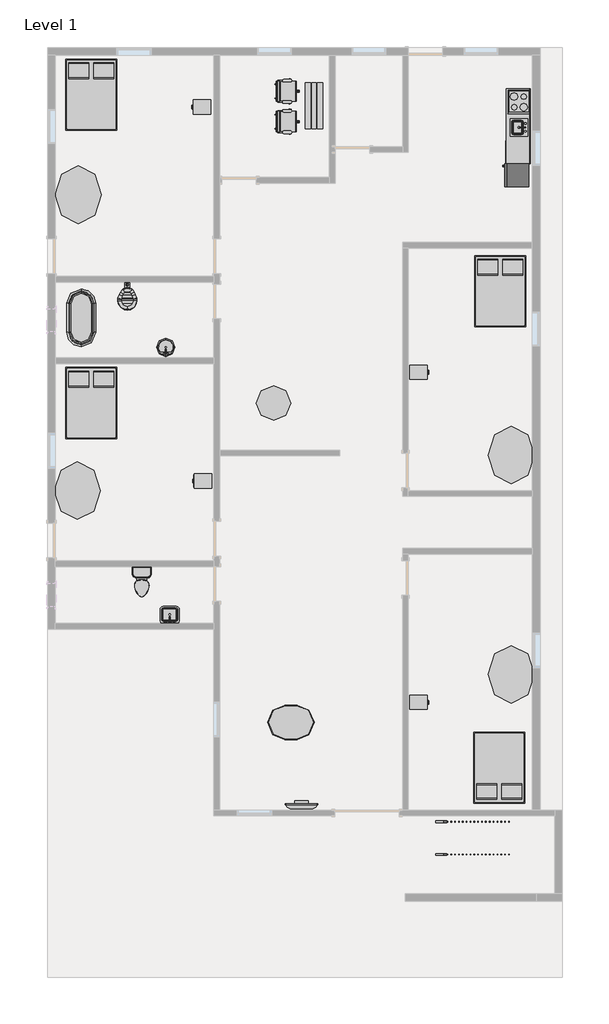
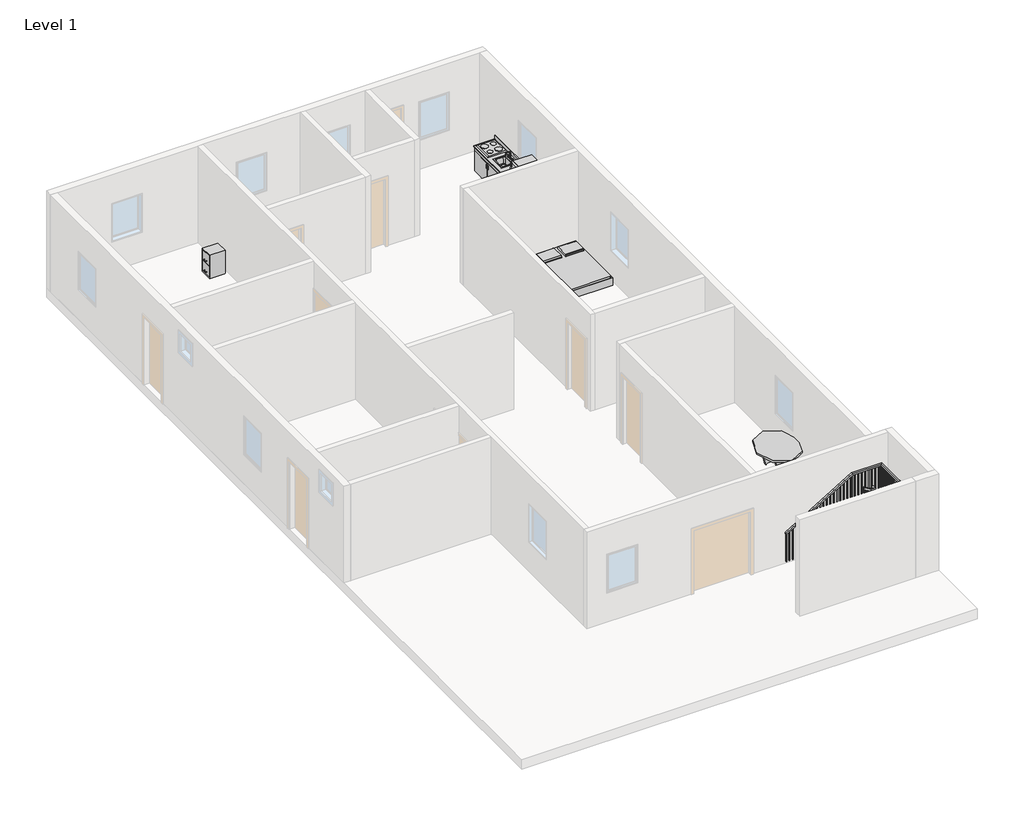
# One storey, part 2 of 2: 19 furniture elements, 6 flow terminals, 4 proxies, 2 railings.
"""IFC4 building model written with IfcOpenShell, lengths in millimetres."""

from ifc_helpers import new_model, si_unit, frame, origin, place, context, project, spatial, polyline, outline, extrude, faceted_brep, transform, mapped, element, save
from components import proxy_a6faaae8, proxy_45b28599, kitchenette_medium_kitchenette_medium_844211aa, proxy_c523a7b7, flow_terminal_871c2e40, flow_terminal_d49f872f, flow_terminal_62a433f7, flow_terminal_6d55091a, toilet_domestic_3d_toilet_domestic_3d_f7549cf7, toilet_domestic_3d_toilet_domestic_3d_183bbd19, flow_terminal_b374fae2, furniture_c8abb964, furniture_39ce88ff, furniture_bb55ed6b, chair_task_arms_chair_task_arms_fa5a08ef, furniture_c6510c7c, furniture_56245f3a, furniture_be1c6672, furniture_905aceb5, furniture_743965d2

model = new_model("IFC4")

# Units and contexts
model_context = context("Model", 3, world=origin())
ifc_project = project(units=[si_unit("LENGTHUNIT", "METRE", prefix="MILLI")], contexts=[model_context])

# Site, building, storey
site = spatial("IfcSite", under=ifc_project)
building = spatial("IfcBuilding", under=site)
storey = spatial("IfcBuildingStorey", under=building, Name="Level 1", Elevation=0.0)

# Proxies
placement = place(None, origin())
proxy_shape = proxy_a6faaae8(model_context)
element("IfcBuildingElementProxy", 1, Name="Cook Top-4 Unit2 : 22\" x 20\"", ObjectType="Cook Top-4 Unit2 : 22\" x 20\"", at=placement, inside=storey, context=model_context, shape_type="MappedRepresentation", body=[
    mapped(proxy_shape, transform((-6479.5409023, 9539.2226537, 0.0), x_axis=(0.0, -1.0000000000000002, 0.0), y_axis=(1.0000000000000002, 0.0, 0.0), z_axis=(0.0, 0.0, 1.0))),
])
proxy_2_shape = proxy_45b28599(model_context)
element("IfcBuildingElementProxy", 2, Name="Dishwasher : 24\" x 24\" x 34\"", ObjectType="Dishwasher : 24\" x 24\" x 34\"", at=placement, inside=storey, context=model_context, shape_type="MappedRepresentation", body=[
    mapped(proxy_2_shape, transform((-6771.3904671, 8588.0401222, 0.0), x_axis=(0.0, -1.0000000000000002, 0.0), y_axis=(1.0000000000000002, 0.0, 0.0), z_axis=(0.0, 0.0, 1.0))),
])
kitchenette_medium_kitchenette_medium_shape = kitchenette_medium_kitchenette_medium_844211aa(model_context)
element("IfcBuildingElementProxy", 3, Name="Kitchenette - Medium : Kitchenette - Medium", ObjectType="Kitchenette - Medium : Kitchenette - Medium", at=placement, inside=storey, context=model_context, shape_type="MappedRepresentation", body=[
    mapped(kitchenette_medium_kitchenette_medium_shape, transform((-6174.7409023, 9215.0603586, 0.0), x_axis=(0.0, -1.0000000000000002, 0.0), y_axis=(1.0000000000000002, 0.0, 0.0), z_axis=(0.0, 0.0, 1.0))),
])
proxy_3_shape = proxy_c523a7b7(model_context)
element("IfcBuildingElementProxy", 4, Name="Refrigerator : 24\" x 25\" LH", ObjectType="Refrigerator : 24\" x 25\" LH", at=placement, inside=storey, context=model_context, shape_type="MappedRepresentation", body=[
    mapped(proxy_3_shape, transform((-6525.1898738, 7602.4726537, 0.0), x_axis=(0.0, -1.0000000000000002, 0.0), y_axis=(1.0000000000000002, 0.0, 0.0), z_axis=(0.0, 0.0, 1.0))),
])

# Flow terminals
flow_terminal_shape = flow_terminal_871c2e40(model_context)
element("IfcFlowTerminal", 5, ObjectType="Sink Kitchen-Island : 18\" x 18\"", at=placement, inside=storey, context=model_context, shape_type="MappedRepresentation", body=[
    mapped(flow_terminal_shape, transform((-6481.8863034, 8881.8118943, -14.4), x_axis=(0.0, -1.0000000000000002, 0.0), y_axis=(1.0000000000000002, 0.0, 0.0), z_axis=(0.0, 0.0, 1.0))),
])
flow_terminal_2_shape = flow_terminal_d49f872f(model_context)
element("IfcFlowTerminal", 6, ObjectType="Sink Vanity-Round : 19\" x 19\"", at=placement, inside=storey, context=model_context, shape_type="MappedRepresentation", body=[
    mapped(flow_terminal_2_shape, transform((-15704.6891617, 3141.6158949, 0.0), x_axis=(-1.0000000000000004, 0.0, 0.0), y_axis=(0.0, -1.0000000000000004, 0.0), z_axis=(0.0, 0.0, 1.0))),
])
flow_terminal_3_shape = flow_terminal_62a433f7(model_context)
element("IfcFlowTerminal", 7, ObjectType="Sink Vanity-Square : 20\" x 18\"", at=placement, inside=storey, context=model_context, shape_type="MappedRepresentation", body=[
    mapped(flow_terminal_3_shape, transform((-15684.0516617, -4048.8679551, 0.0), x_axis=(-1.0000000000000002, 0.0, 0.0), y_axis=(0.0, -1.0000000000000002, 0.0), z_axis=(0.0, 0.0, 1.0))),
])
flow_terminal_4_shape = flow_terminal_6d55091a(model_context)
element("IfcFlowTerminal", 8, ObjectType="Toilet-Commercial-Wall-3D : 15\" Seat Height", at=placement, inside=storey, context=model_context, shape_type="MappedRepresentation", body=[
    mapped(flow_terminal_4_shape, transform((-16412.4377485, 4852.9226537, 0.0), x_axis=(-1.0, 0.0, 0.0), y_axis=(0.0, -1.0, 0.0), z_axis=(0.0, 0.0, 1.0))),
])
toilet_domestic_3d_toilet_domestic_3d_shape = toilet_domestic_3d_toilet_domestic_3d_f7549cf7(model_context)
toilet_domestic_3d_toilet_domestic_3d_2_shape = toilet_domestic_3d_toilet_domestic_3d_183bbd19(model_context)
element("IfcFlowTerminal", 9, ObjectType="Toilet-Domestic-3D : Toilet-Domestic-3D", at=placement, inside=storey, context=model_context, shape_type="MappedRepresentation", body=[
    mapped(toilet_domestic_3d_toilet_domestic_3d_shape, transform((-16436.3409023, -3225.1093836, 0.0), x_axis=(1.0, 0.0, 0.0), y_axis=(0.0, 1.0, 0.0), z_axis=(0.0, 0.0, 1.0))),
    mapped(toilet_domestic_3d_toilet_domestic_3d_2_shape, transform((-16436.3409023, -3225.1093836, 0.0), x_axis=(1.0, 0.0, 0.0), y_axis=(0.0, 1.0, 0.0), z_axis=(0.0, 0.0, 1.0))),
])
flow_terminal_5_shape = flow_terminal_b374fae2(model_context)
element("IfcFlowTerminal", 10, ObjectType="Tub-Free Standing-3D : 30\" x 60\"", at=placement, inside=storey, context=model_context, shape_type="MappedRepresentation", body=[
    mapped(flow_terminal_5_shape, transform((-18036.5409023, 3836.9226537, 0.0), x_axis=(1.0, 0.0, 0.0), y_axis=(0.0, 1.0, 0.0), z_axis=(0.0, 0.0, 1.0))),
])

# Furniture
furniture_shape = furniture_c8abb964(model_context)
element("IfcFurniture", 11, ObjectType="Bed-Box : Double 53\" x 74\"", at=placement, inside=storey, context=model_context, shape_type="MappedRepresentation", body=[
    mapped(furniture_shape, transform((-18108.9933613, 9964.1521619, 0.0), x_axis=(1.0, 0.0, 0.0), y_axis=(0.0, 1.0, 0.0), z_axis=(0.0, 0.0, 1.0))),
])
element("IfcFurniture", 12, ObjectType="Bed-Box : Double 53\" x 74\"", at=placement, inside=storey, context=model_context, shape_type="MappedRepresentation", body=[
    mapped(furniture_shape, transform((-18108.9933613, 1822.016152, 0.0), x_axis=(1.0, 0.0, 0.0), y_axis=(0.0, 1.0, 0.0), z_axis=(0.0, 0.0, 1.0))),
])
element("IfcFurniture", 13, ObjectType="Bed-Box : Double 53\" x 74\"", at=placement, inside=storey, context=model_context, shape_type="MappedRepresentation", body=[
    mapped(furniture_shape, transform((-7313.9933613, 4776.7226537, 0.0), x_axis=(1.0, 0.0, 0.0), y_axis=(0.0, 1.0, 0.0), z_axis=(0.0, 0.0, 1.0))),
])
element("IfcFurniture", 14, ObjectType="Bed-Box : Double 53\" x 74\"", at=placement, inside=storey, context=model_context, shape_type="MappedRepresentation", body=[
    mapped(furniture_shape, transform((-6661.0884433, -8273.4428644, 0.0), x_axis=(-1.0000000000000002, 0.0, 0.0), y_axis=(0.0, -1.0000000000000002, 0.0), z_axis=(0.0, 0.0, 1.0))),
])
furniture_2_shape = furniture_39ce88ff(model_context)
element("IfcFurniture", 15, ObjectType="Bench-Locker Room : 48\" x 18\" x 14\"", at=placement, inside=storey, context=model_context, shape_type="MappedRepresentation", body=[
    mapped(furniture_2_shape, transform((-11709.0261482, 9282.3078996, 0.0), x_axis=(0.0, -1.0000000000000002, 0.0), y_axis=(1.0000000000000002, 0.0, 0.0), z_axis=(0.0, 0.0, 1.0))),
])
furniture_3_shape = furniture_bb55ed6b(model_context)
element("IfcFurniture", 16, ObjectType="Cabinet-File 2 Drawer : 15\" x 18\"", at=placement, inside=storey, context=model_context, shape_type="MappedRepresentation", body=[
    mapped(furniture_3_shape, transform((-14706.7066022, 9271.6262067, 0.0), x_axis=(0.0, -1.0000000000000007, 0.0), y_axis=(1.0000000000000007, 0.0, 0.0), z_axis=(0.0, 0.0, 1.0))),
])
element("IfcFurniture", 17, ObjectType="Cabinet-File 2 Drawer : 15\" x 18\"", at=placement, inside=storey, context=model_context, shape_type="MappedRepresentation", body=[
    mapped(furniture_3_shape, transform((-14681.3066022, -597.7098032, 0.0), x_axis=(0.0, -1.0000000000000007, 0.0), y_axis=(1.0000000000000007, 0.0, 0.0), z_axis=(0.0, 0.0, 1.0))),
])
element("IfcFurniture", 18, ObjectType="Cabinet-File 2 Drawer : 15\" x 18\"", at=placement, inside=storey, context=model_context, shape_type="MappedRepresentation", body=[
    mapped(furniture_3_shape, transform((-9275.9752024, 2528.2830908, 0.0), x_axis=(0.0, 1.0000000000000002, 0.0), y_axis=(-1.0000000000000002, 0.0, 0.0), z_axis=(0.0, 0.0, 1.0))),
])
element("IfcFurniture", 19, ObjectType="Cabinet-File 2 Drawer : 15\" x 18\"", at=placement, inside=storey, context=model_context, shape_type="MappedRepresentation", body=[
    mapped(furniture_3_shape, transform((-9275.9752024, -6183.9169092, 0.0), x_axis=(0.0, 1.000000000000001, 0.0), y_axis=(-1.000000000000001, 0.0, 0.0), z_axis=(0.0, 0.0, 1.0))),
])
chair_task_arms_chair_task_arms_shape = chair_task_arms_chair_task_arms_fa5a08ef(model_context)
element("IfcFurniture", 20, ObjectType="Chair-Task Arms : Chair-Task Arms", at=placement, inside=storey, context=model_context, shape_type="MappedRepresentation", body=[
    mapped(chair_task_arms_chair_task_arms_shape, transform((-12645.2868039, 9959.6134734, 0.0), x_axis=(0.0, -1.0000000000000004, 0.0), y_axis=(1.0000000000000004, 0.0, 0.0), z_axis=(0.0, 0.0, 1.0))),
])
element("IfcFurniture", 21, ObjectType="Chair-Task Arms : Chair-Task Arms", at=placement, inside=storey, context=model_context, shape_type="MappedRepresentation", body=[
    mapped(chair_task_arms_chair_task_arms_shape, transform((-12645.2868039, 9159.5134734, 0.0), x_axis=(0.0, -1.0000000000000004, 0.0), y_axis=(1.0000000000000004, 0.0, 0.0), z_axis=(0.0, 0.0, 1.0))),
])
furniture_4_shape = furniture_c6510c7c(model_context)
element("IfcFurniture", 22, ObjectType="Counter Top w Sink Hole : 24\" Depth", at=placement, inside=storey, context=model_context, shape_type="MappedRepresentation", body=[
    mapped(furniture_4_shape, transform((-6174.7409023, 8681.6603586, -14.4), x_axis=(0.0, -1.0000000000000002, 0.0), y_axis=(1.0000000000000002, 0.0, 0.0), z_axis=(0.0, 0.0, 1.0))),
])
furniture_5_shape = furniture_56245f3a(model_context)
element("IfcFurniture", 23, ObjectType="TV - Flat Screen : 32\"", at=placement, inside=storey, context=model_context, shape_type="MappedRepresentation", body=[
    mapped(furniture_5_shape, transform((-12223.8854164, -9063.1108623, 0.0), x_axis=(-1.000000000000001, 0.0, 0.0), y_axis=(0.0, -1.000000000000001, 0.0), z_axis=(0.0, 0.0, 1.0))),
])
furniture_6_shape = furniture_be1c6672(model_context)
element("IfcFurniture", 24, ObjectType="Table-Dining Oval : 36\" x 48\"", at=placement, inside=storey, context=model_context, shape_type="MappedRepresentation", body=[
    mapped(furniture_6_shape, transform((-12097.5212302, -6487.1149956, 0.0), x_axis=(1.0, 0.0, 0.0), y_axis=(0.0, 1.0, 0.0), z_axis=(0.0, 0.0, 1.0))),
])
furniture_7_shape = furniture_905aceb5(model_context)
element("IfcFurniture", 25, ObjectType="Table-Dining Round w Chairs : 36\" Diameter", at=placement, inside=storey, context=model_context, shape_type="MappedRepresentation", body=[
    mapped(furniture_7_shape, transform((-13060.2228695, 1772.4653323, 0.0), x_axis=(1.0, 0.0, 0.0), y_axis=(0.0, 1.0, 0.0), z_axis=(0.0, 0.0, 1.0))),
])
furniture_8_shape = furniture_743965d2(model_context)
element("IfcFurniture", 26, ObjectType="Table-Ellipse : 60\" x 48\"", at=placement, inside=storey, context=model_context, shape_type="MappedRepresentation", body=[
    mapped(furniture_8_shape, transform((-18112.7409023, 7088.1226537, 0.0), x_axis=(0.0, 1.0000000000000002, 0.0), y_axis=(-1.0000000000000002, 0.0, 0.0), z_axis=(0.0, 0.0, 1.0))),
])
element("IfcFurniture", 27, ObjectType="Table-Ellipse : 60\" x 48\"", at=placement, inside=storey, context=model_context, shape_type="MappedRepresentation", body=[
    mapped(furniture_8_shape, transform((-18138.1409023, -723.8133562, 0.0), x_axis=(0.0, 1.0000000000000002, 0.0), y_axis=(-1.0000000000000002, 0.0, 0.0), z_axis=(0.0, 0.0, 1.0))),
])
element("IfcFurniture", 28, ObjectType="Table-Ellipse : 60\" x 48\"", at=placement, inside=storey, context=model_context, shape_type="MappedRepresentation", body=[
    mapped(furniture_8_shape, transform((-6682.7409023, 215.9866438, 0.0), x_axis=(0.0, -1.0000000000000004, 0.0), y_axis=(1.0000000000000004, 0.0, 0.0), z_axis=(0.0, 0.0, 1.0))),
])
element("IfcFurniture", 29, ObjectType="Table-Ellipse : 60\" x 48\"", at=placement, inside=storey, context=model_context, shape_type="MappedRepresentation", body=[
    mapped(furniture_8_shape, transform((-6682.7409023, -5575.2133562, 0.0), x_axis=(0.0, -1.0, 0.0), y_axis=(1.0, 0.0, 0.0), z_axis=(0.0, 0.0, 1.0))),
])

# Railings
element("IfcRailing", 30, ObjectType="Handrail - Rectangular", at=placement, inside=storey, context=model_context, shape_type="SolidModel", body=[
    faceted_brep([(-8674.4712983, -10304.6989716, 1083.7333333), (-8674.4712983, -10304.6989716, 1024.3318731), (-8674.4712983, -10355.4989716, 1024.3318731), (-8674.4712983, -10355.4989716, 1083.7333333), (-6794.8712983, -10304.6989716, 2222.8848485), (-6744.0712983, -10304.6989716, 2194.271267), (-6744.0712983, -10355.4989716, 2194.271267), (-6794.8712983, -10355.4989716, 2222.8848485), (-6794.8712983, -10304.6989716, 2269.0666667), (-6744.0712983, -10304.6989716, 2218.2666667), (-6744.0712983, -10355.4989716, 2218.2666667), (-6794.8712983, -10355.4989716, 2269.0666667), (-6667.8712983, -10304.6989716, 2269.0666667), (-6667.8712983, -10304.6989716, 2218.2666667), (-6718.6712983, -10355.4989716, 2218.2666667), (-6718.6712983, -10355.4989716, 2269.0666667), (-6667.8712983, -10431.6989716, 2269.0666667), (-6667.8712983, -10431.6989716, 2218.2666667), (-6718.6712983, -10431.6989716, 2218.2666667), (-6718.6712983, -10431.6989716, 2269.0666667), (-6667.8712983, -10491.4341545, 2269.0666667), (-6667.8712983, -10542.2341545, 2218.2666667), (-6718.6712983, -10542.2341545, 2218.2666667), (-6718.6712983, -10491.4341545, 2269.0666667), (-6667.8712983, -10491.4341545, 2484.5818182), (-6667.8712983, -10542.2341545, 2433.7818182), (-6718.6712983, -10542.2341545, 2433.7818182), (-6718.6712983, -10491.4341545, 2484.5818182), (-6667.8712983, -10618.4341545, 2484.5818182), (-6667.8712983, -10618.4341545, 2433.7818182), (-6718.6712983, -10567.6341545, 2433.7818182), (-6718.6712983, -10567.6341545, 2484.5818182), (-6794.8712983, -10618.4341545, 2484.5818182), (-6809.0637077, -10618.4341545, 2433.7818182), (-6809.0637077, -10567.6341545, 2433.7818182), (-6794.8712983, -10567.6341545, 2484.5818182), (-6998.0712983, -10618.4341545, 2607.7333333), (-6998.0712983, -10567.6341545, 2607.7333333), (-6998.0712983, -10567.6341545, 2548.3318731), (-6998.0712983, -10618.4341545, 2548.3318731)], [[[0, 1, 2, 3]], [[1, 0, 4, 5]], [[2, 1, 5, 6]], [[3, 2, 6, 7]], [[0, 3, 7, 4]], [[5, 4, 8, 9]], [[6, 5, 9, 10]], [[7, 6, 10, 11]], [[4, 7, 11, 8]], [[9, 8, 12, 13]], [[10, 9, 13, 14]], [[11, 10, 14, 15]], [[8, 11, 15, 12]], [[13, 12, 16, 17]], [[14, 13, 17, 18]], [[15, 14, 18, 19]], [[12, 15, 19, 16]], [[17, 16, 20, 21]], [[18, 17, 21, 22]], [[19, 18, 22, 23]], [[16, 19, 23, 20]], [[21, 20, 24, 25]], [[22, 21, 25, 26]], [[23, 22, 26, 27]], [[20, 23, 27, 24]], [[25, 24, 28, 29]], [[26, 25, 29, 30]], [[27, 26, 30, 31]], [[24, 27, 31, 28]], [[29, 28, 32, 33]], [[30, 29, 33, 34]], [[31, 30, 34, 35]], [[28, 31, 35, 32]], [[36, 37, 38, 39]], [[33, 32, 36, 39]], [[34, 33, 39, 38]], [[35, 34, 38, 37]], [[32, 35, 37, 36]]]),
    extrude(outline(polyline([(2480.9833882, -6886.9462983), (2492.5288428, -6905.9962983), (1524.0, -6905.9962983), (1524.0, -6886.9462983), (2480.9833882, -6886.9462983)])), frame((0.0, -10602.5591545, 0.0), z_axis=(0.0, 1.0, 0.0), x_axis=(0.0, 0.0, 1.0)), (0.0, 0.0, 1.0), 19.05),
    extrude(outline(polyline([(-6785.3462983, -10583.5091545), (-6785.3462983, -10602.5591545), (-6804.3962983, -10602.5591545), (-6804.3962983, -10583.5091545), (-6785.3462983, -10583.5091545)])), frame((0.0, 0.0, 1524.0), z_axis=(0.0, 0.0, 1.0), x_axis=(1.0, 0.0, 0.0)), (0.0, 0.0, 1.0), 909.7818182),
    extrude(outline(polyline([(-6702.7962983, -10523.7739716), (-6683.7462983, -10523.7739716), (-6683.7462983, -10542.8239716), (-6702.7962983, -10542.8239716), (-6702.7962983, -10523.7739716)])), frame((0.0, 0.0, 1354.6666667), z_axis=(0.0, 0.0, 1.0), x_axis=(1.0, 0.0, 0.0)), (0.0, 0.0, 1.0), 863.6),
    extrude(outline(polyline([(-6702.7962983, -10422.1739716), (-6683.7462983, -10422.1739716), (-6683.7462983, -10441.2239716), (-6702.7962983, -10441.2239716), (-6702.7962983, -10422.1739716)])), frame((0.0, 0.0, 1354.6666667), z_axis=(0.0, 0.0, 1.0), x_axis=(1.0, 0.0, 0.0)), (0.0, 0.0, 1.0), 863.6),
    extrude(outline(polyline([(2200.0439943, -6734.5462983), (2188.4985397, -6753.5962983), (1185.3333333, -6753.5962983), (1185.3333333, -6734.5462983), (2200.0439943, -6734.5462983)])), frame((0.0, -10339.6239716, 0.0), z_axis=(0.0, 1.0, 0.0), x_axis=(0.0, 0.0, 1.0)), (0.0, 0.0, 1.0), 19.05),
    extrude(outline(polyline([(2138.4682367, -6836.1462983), (2126.9227822, -6855.1962983), (1185.3333333, -6855.1962983), (1185.3333333, -6836.1462983), (2138.4682367, -6836.1462983)])), frame((0.0, -10339.6239716, 0.0), z_axis=(0.0, 1.0, 0.0), x_axis=(0.0, 0.0, 1.0)), (0.0, 0.0, 1.0), 19.05),
    extrude(outline(polyline([(2076.8924791, -6937.7462983), (2065.3470246, -6956.7962983), (1185.3333333, -6956.7962983), (1185.3333333, -6937.7462983), (2076.8924791, -6937.7462983)])), frame((0.0, -10339.6239716, 0.0), z_axis=(0.0, 1.0, 0.0), x_axis=(0.0, 0.0, 1.0)), (0.0, 0.0, 1.0), 19.05),
    extrude(outline(polyline([(2015.3167216, -7039.3462983), (2003.771267, -7058.3962983), (1016.0, -7058.3962983), (1016.0, -7039.3462983), (2015.3167216, -7039.3462983)])), frame((0.0, -10339.6239716, 0.0), z_axis=(0.0, 1.0, 0.0), x_axis=(0.0, 0.0, 1.0)), (0.0, 0.0, 1.0), 19.05),
    extrude(outline(polyline([(1953.740964, -7140.9462983), (1942.1955094, -7159.9962983), (1016.0, -7159.9962983), (1016.0, -7140.9462983), (1953.740964, -7140.9462983)])), frame((0.0, -10339.6239716, 0.0), z_axis=(0.0, 1.0, 0.0), x_axis=(0.0, 0.0, 1.0)), (0.0, 0.0, 1.0), 19.05),
    extrude(outline(polyline([(1892.1652064, -7242.5462983), (1880.6197519, -7261.5962983), (1016.0, -7261.5962983), (1016.0, -7242.5462983), (1892.1652064, -7242.5462983)])), frame((0.0, -10339.6239716, 0.0), z_axis=(0.0, 1.0, 0.0), x_axis=(0.0, 0.0, 1.0)), (0.0, 0.0, 1.0), 19.05),
    extrude(outline(polyline([(1830.5894488, -7344.1462983), (1819.0439943, -7363.1962983), (846.6666667, -7363.1962983), (846.6666667, -7344.1462983), (1830.5894488, -7344.1462983)])), frame((0.0, -10339.6239716, 0.0), z_axis=(0.0, 1.0, 0.0), x_axis=(0.0, 0.0, 1.0)), (0.0, 0.0, 1.0), 19.05),
    extrude(outline(polyline([(1769.0136913, -7445.7462983), (1757.4682367, -7464.7962983), (846.6666667, -7464.7962983), (846.6666667, -7445.7462983), (1769.0136913, -7445.7462983)])), frame((0.0, -10339.6239716, 0.0), z_axis=(0.0, 1.0, 0.0), x_axis=(0.0, 0.0, 1.0)), (0.0, 0.0, 1.0), 19.05),
    extrude(outline(polyline([(1707.4379337, -7547.3462983), (1695.8924791, -7566.3962983), (846.6666667, -7566.3962983), (846.6666667, -7547.3462983), (1707.4379337, -7547.3462983)])), frame((0.0, -10339.6239716, 0.0), z_axis=(0.0, 1.0, 0.0), x_axis=(0.0, 0.0, 1.0)), (0.0, 0.0, 1.0), 19.05),
    extrude(outline(polyline([(1645.8621761, -7648.9462983), (1634.3167216, -7667.9962983), (677.3333333, -7667.9962983), (677.3333333, -7648.9462983), (1645.8621761, -7648.9462983)])), frame((0.0, -10339.6239716, 0.0), z_axis=(0.0, 1.0, 0.0), x_axis=(0.0, 0.0, 1.0)), (0.0, 0.0, 1.0), 19.05),
    extrude(outline(polyline([(1584.2864185, -7750.5462983), (1572.740964, -7769.5962983), (677.3333333, -7769.5962983), (677.3333333, -7750.5462983), (1584.2864185, -7750.5462983)])), frame((0.0, -10339.6239716, 0.0), z_axis=(0.0, 1.0, 0.0), x_axis=(0.0, 0.0, 1.0)), (0.0, 0.0, 1.0), 19.05),
    extrude(outline(polyline([(1522.710661, -7852.1462983), (1511.1652064, -7871.1962983), (508.0, -7871.1962983), (508.0, -7852.1462983), (1522.710661, -7852.1462983)])), frame((0.0, -10339.6239716, 0.0), z_axis=(0.0, 1.0, 0.0), x_axis=(0.0, 0.0, 1.0)), (0.0, 0.0, 1.0), 19.05),
    extrude(outline(polyline([(1461.1349034, -7953.7462983), (1449.5894488, -7972.7962983), (508.0, -7972.7962983), (508.0, -7953.7462983), (1461.1349034, -7953.7462983)])), frame((0.0, -10339.6239716, 0.0), z_axis=(0.0, 1.0, 0.0), x_axis=(0.0, 0.0, 1.0)), (0.0, 0.0, 1.0), 19.05),
    extrude(outline(polyline([(1399.5591458, -8055.3462983), (1388.0136913, -8074.3962983), (508.0, -8074.3962983), (508.0, -8055.3462983), (1399.5591458, -8055.3462983)])), frame((0.0, -10339.6239716, 0.0), z_axis=(0.0, 1.0, 0.0), x_axis=(0.0, 0.0, 1.0)), (0.0, 0.0, 1.0), 19.05),
    extrude(outline(polyline([(1337.9833882, -8156.9462983), (1326.4379337, -8175.9962983), (338.6666667, -8175.9962983), (338.6666667, -8156.9462983), (1337.9833882, -8156.9462983)])), frame((0.0, -10339.6239716, 0.0), z_axis=(0.0, 1.0, 0.0), x_axis=(0.0, 0.0, 1.0)), (0.0, 0.0, 1.0), 19.05),
    extrude(outline(polyline([(1276.4076307, -8258.5462983), (1264.8621761, -8277.5962983), (338.6666667, -8277.5962983), (338.6666667, -8258.5462983), (1276.4076307, -8258.5462983)])), frame((0.0, -10339.6239716, 0.0), z_axis=(0.0, 1.0, 0.0), x_axis=(0.0, 0.0, 1.0)), (0.0, 0.0, 1.0), 19.05),
    extrude(outline(polyline([(1214.8318731, -8360.1462983), (1203.2864185, -8379.1962983), (338.6666667, -8379.1962983), (338.6666667, -8360.1462983), (1214.8318731, -8360.1462983)])), frame((0.0, -10339.6239716, 0.0), z_axis=(0.0, 1.0, 0.0), x_axis=(0.0, 0.0, 1.0)), (0.0, 0.0, 1.0), 19.05),
    extrude(outline(polyline([(1153.2561155, -8461.7462983), (1141.710661, -8480.7962983), (169.3333333, -8480.7962983), (169.3333333, -8461.7462983), (1153.2561155, -8461.7462983)])), frame((0.0, -10339.6239716, 0.0), z_axis=(0.0, 1.0, 0.0), x_axis=(0.0, 0.0, 1.0)), (0.0, 0.0, 1.0), 19.05),
    extrude(outline(polyline([(1091.6803579, -8563.3462983), (1080.1349034, -8582.3962983), (169.3333333, -8582.3962983), (169.3333333, -8563.3462983), (1091.6803579, -8563.3462983)])), frame((0.0, -10339.6239716, 0.0), z_axis=(0.0, 1.0, 0.0), x_axis=(0.0, 0.0, 1.0)), (0.0, 0.0, 1.0), 19.05),
    extrude(outline(polyline([(-6683.7462983, -10583.5091545), (-6683.7462983, -10602.5591545), (-6702.7962983, -10602.5591545), (-6702.7962983, -10583.5091545), (-6683.7462983, -10583.5091545)])), frame((0.0, 0.0, 1354.6666667), z_axis=(0.0, 0.0, 1.0), x_axis=(1.0, 0.0, 0.0)), (0.0, 0.0, 1.0), 1079.1151515),
    extrude(outline(polyline([(-6702.7962983, -10339.6239716), (-6702.7962983, -10320.5739716), (-6683.7462983, -10320.5739716), (-6683.7462983, -10339.6239716), (-6702.7962983, -10339.6239716)])), frame((0.0, 0.0, 1354.6666667), z_axis=(0.0, 0.0, 1.0), x_axis=(1.0, 0.0, 0.0)), (0.0, 0.0, 1.0), 863.6),
    extrude(outline(polyline([(-6728.1962983, -10339.6239716), (-6728.1962983, -10320.5739716), (-6709.1462983, -10320.5739716), (-6709.1462983, -10339.6239716), (-6728.1962983, -10339.6239716)])), frame((0.0, 0.0, 1354.6666667), z_axis=(0.0, 0.0, 1.0), x_axis=(1.0, 0.0, 0.0)), (0.0, 0.0, 1.0), 863.6),
    extrude(outline(polyline([(2536.7864185, -6979.0212983), (2548.3318731, -6998.0712983), (1524.0, -6998.0712983), (1524.0, -6979.0212983), (2536.7864185, -6979.0212983)])), frame((0.0, -10602.5591545, 0.0), z_axis=(0.0, 1.0, 0.0), x_axis=(0.0, 0.0, 1.0)), (0.0, 0.0, 1.0), 19.05),
    extrude(outline(polyline([(1035.8773276, -8655.4212983), (1024.3318731, -8674.4712983), (169.3333333, -8674.4712983), (169.3333333, -8655.4212983), (1035.8773276, -8655.4212983)])), frame((0.0, -10339.6239716, 0.0), z_axis=(0.0, 1.0, 0.0), x_axis=(0.0, 0.0, 1.0)), (0.0, 0.0, 1.0), 19.05),
])
element("IfcRailing", 31, ObjectType="Handrail - Rectangular", at=placement, inside=storey, context=model_context, shape_type="SolidModel", body=[
    faceted_brep([(-8674.4712983, -9441.0989716, 1083.7333333), (-8674.4712983, -9441.0989716, 1024.3318731), (-8674.4712983, -9491.8989716, 1024.3318731), (-8674.4712983, -9491.8989716, 1083.7333333), (-6718.6712983, -9441.0989716, 2269.0666667), (-6704.4788889, -9441.0989716, 2218.2666667), (-6704.4788889, -9491.8989716, 2218.2666667), (-6718.6712983, -9491.8989716, 2269.0666667), (-5804.2712983, -9441.0989716, 2269.0666667), (-5804.2712983, -9441.0989716, 2218.2666667), (-5855.0712983, -9491.8989716, 2218.2666667), (-5855.0712983, -9491.8989716, 2269.0666667), (-5804.2712983, -11228.0341545, 2269.0666667), (-5804.2712983, -11228.0341545, 2218.2666667), (-5855.0712983, -11177.2341545, 2218.2666667), (-5855.0712983, -11177.2341545, 2269.0666667), (-6439.2712983, -11228.0341545, 2269.0666667), (-6453.4637077, -11228.0341545, 2218.2666667), (-6453.4637077, -11177.2341545, 2218.2666667), (-6439.2712983, -11177.2341545, 2269.0666667), (-6998.0712983, -11228.0341545, 2607.7333333), (-6998.0712983, -11177.2341545, 2607.7333333), (-6998.0712983, -11177.2341545, 2548.3318731), (-6998.0712983, -11228.0341545, 2548.3318731)], [[[0, 1, 2, 3]], [[1, 0, 4, 5]], [[2, 1, 5, 6]], [[3, 2, 6, 7]], [[0, 3, 7, 4]], [[5, 4, 8, 9]], [[6, 5, 9, 10]], [[7, 6, 10, 11]], [[4, 7, 11, 8]], [[9, 8, 12, 13]], [[10, 9, 13, 14]], [[11, 10, 14, 15]], [[8, 11, 15, 12]], [[13, 12, 16, 17]], [[14, 13, 17, 18]], [[15, 14, 18, 19]], [[12, 15, 19, 16]], [[20, 21, 22, 23]], [[17, 16, 20, 23]], [[18, 17, 23, 22]], [[19, 18, 22, 21]], [[16, 19, 21, 20]]]),
    extrude(outline(polyline([(2523.3167216, -6956.7962983), (1524.0, -6956.7962983), (1524.0, -6937.7462983), (2511.771267, -6937.7462983), (2523.3167216, -6956.7962983)])), frame((0.0, -11212.1591545, 0.0), z_axis=(0.0, 1.0, 0.0), x_axis=(0.0, 0.0, 1.0)), (0.0, 0.0, 1.0), 19.05),
    extrude(outline(polyline([(2461.740964, -6855.1962983), (1524.0, -6855.1962983), (1524.0, -6836.1462983), (2450.1955094, -6836.1462983), (2461.740964, -6855.1962983)])), frame((0.0, -11212.1591545, 0.0), z_axis=(0.0, 1.0, 0.0), x_axis=(0.0, 0.0, 1.0)), (0.0, 0.0, 1.0), 19.05),
    extrude(outline(polyline([(2400.1652064, -6753.5962983), (1524.0, -6753.5962983), (1524.0, -6734.5462983), (2388.6197519, -6734.5462983), (2400.1652064, -6753.5962983)])), frame((0.0, -11212.1591545, 0.0), z_axis=(0.0, 1.0, 0.0), x_axis=(0.0, 0.0, 1.0)), (0.0, 0.0, 1.0), 19.05),
    extrude(outline(polyline([(2338.5894488, -6651.9962983), (1354.6666667, -6651.9962983), (1354.6666667, -6632.9462983), (2327.0439943, -6632.9462983), (2338.5894488, -6651.9962983)])), frame((0.0, -11212.1591545, 0.0), z_axis=(0.0, 1.0, 0.0), x_axis=(0.0, 0.0, 1.0)), (0.0, 0.0, 1.0), 19.05),
    extrude(outline(polyline([(2277.0136913, -6550.3962983), (1354.6666667, -6550.3962983), (1354.6666667, -6531.3462983), (2265.4682367, -6531.3462983), (2277.0136913, -6550.3962983)])), frame((0.0, -11212.1591545, 0.0), z_axis=(0.0, 1.0, 0.0), x_axis=(0.0, 0.0, 1.0)), (0.0, 0.0, 1.0), 19.05),
    extrude(outline(polyline([(-6328.1462983, -11212.1591545), (-6347.1962983, -11212.1591545), (-6347.1962983, -11193.1091545), (-6328.1462983, -11193.1091545), (-6328.1462983, -11212.1591545)])), frame((0.0, 0.0, 1354.6666667), z_axis=(0.0, 0.0, 1.0), x_axis=(1.0, 0.0, 0.0)), (0.0, 0.0, 1.0), 863.6),
    extrude(outline(polyline([(-6226.5462983, -11212.1591545), (-6245.5962983, -11212.1591545), (-6245.5962983, -11193.1091545), (-6226.5462983, -11193.1091545), (-6226.5462983, -11212.1591545)])), frame((0.0, 0.0, 1354.6666667), z_axis=(0.0, 0.0, 1.0), x_axis=(1.0, 0.0, 0.0)), (0.0, 0.0, 1.0), 863.6),
    extrude(outline(polyline([(-6124.9462983, -11212.1591545), (-6143.9962983, -11212.1591545), (-6143.9962983, -11193.1091545), (-6124.9462983, -11193.1091545), (-6124.9462983, -11212.1591545)])), frame((0.0, 0.0, 1354.6666667), z_axis=(0.0, 0.0, 1.0), x_axis=(1.0, 0.0, 0.0)), (0.0, 0.0, 1.0), 863.6),
    extrude(outline(polyline([(-6023.3462983, -11212.1591545), (-6042.3962983, -11212.1591545), (-6042.3962983, -11193.1091545), (-6023.3462983, -11193.1091545), (-6023.3462983, -11212.1591545)])), frame((0.0, 0.0, 1354.6666667), z_axis=(0.0, 0.0, 1.0), x_axis=(1.0, 0.0, 0.0)), (0.0, 0.0, 1.0), 863.6),
    extrude(outline(polyline([(-5921.7462983, -11212.1591545), (-5940.7962983, -11212.1591545), (-5940.7962983, -11193.1091545), (-5921.7462983, -11193.1091545), (-5921.7462983, -11212.1591545)])), frame((0.0, 0.0, 1354.6666667), z_axis=(0.0, 0.0, 1.0), x_axis=(1.0, 0.0, 0.0)), (0.0, 0.0, 1.0), 863.6),
    extrude(outline(polyline([(-5820.1462983, -11184.1739716), (-5820.1462983, -11203.2239716), (-5839.1962983, -11203.2239716), (-5839.1962983, -11184.1739716), (-5820.1462983, -11184.1739716)])), frame((0.0, 0.0, 1354.6666667), z_axis=(0.0, 0.0, 1.0), x_axis=(1.0, 0.0, 0.0)), (0.0, 0.0, 1.0), 863.6),
    extrude(outline(polyline([(-5820.1462983, -11082.5739716), (-5820.1462983, -11101.6239716), (-5839.1962983, -11101.6239716), (-5839.1962983, -11082.5739716), (-5820.1462983, -11082.5739716)])), frame((0.0, 0.0, 1354.6666667), z_axis=(0.0, 0.0, 1.0), x_axis=(1.0, 0.0, 0.0)), (0.0, 0.0, 1.0), 863.6),
    extrude(outline(polyline([(-5820.1462983, -10980.9739716), (-5820.1462983, -11000.0239716), (-5839.1962983, -11000.0239716), (-5839.1962983, -10980.9739716), (-5820.1462983, -10980.9739716)])), frame((0.0, 0.0, 1354.6666667), z_axis=(0.0, 0.0, 1.0), x_axis=(1.0, 0.0, 0.0)), (0.0, 0.0, 1.0), 863.6),
    extrude(outline(polyline([(-5820.1462983, -10879.3739716), (-5820.1462983, -10898.4239716), (-5839.1962983, -10898.4239716), (-5839.1962983, -10879.3739716), (-5820.1462983, -10879.3739716)])), frame((0.0, 0.0, 1354.6666667), z_axis=(0.0, 0.0, 1.0), x_axis=(1.0, 0.0, 0.0)), (0.0, 0.0, 1.0), 863.6),
    extrude(outline(polyline([(-5820.1462983, -10777.7739716), (-5820.1462983, -10796.8239716), (-5839.1962983, -10796.8239716), (-5839.1962983, -10777.7739716), (-5820.1462983, -10777.7739716)])), frame((0.0, 0.0, 1354.6666667), z_axis=(0.0, 0.0, 1.0), x_axis=(1.0, 0.0, 0.0)), (0.0, 0.0, 1.0), 863.6),
    extrude(outline(polyline([(-5820.1462983, -10676.1739716), (-5820.1462983, -10695.2239716), (-5839.1962983, -10695.2239716), (-5839.1962983, -10676.1739716), (-5820.1462983, -10676.1739716)])), frame((0.0, 0.0, 1354.6666667), z_axis=(0.0, 0.0, 1.0), x_axis=(1.0, 0.0, 0.0)), (0.0, 0.0, 1.0), 863.6),
    extrude(outline(polyline([(-5820.1462983, -10574.5739716), (-5820.1462983, -10593.6239716), (-5839.1962983, -10593.6239716), (-5839.1962983, -10574.5739716), (-5820.1462983, -10574.5739716)])), frame((0.0, 0.0, 1354.6666667), z_axis=(0.0, 0.0, 1.0), x_axis=(1.0, 0.0, 0.0)), (0.0, 0.0, 1.0), 863.6),
    extrude(outline(polyline([(-5820.1462983, -10472.9739716), (-5820.1462983, -10492.0239716), (-5839.1962983, -10492.0239716), (-5839.1962983, -10472.9739716), (-5820.1462983, -10472.9739716)])), frame((0.0, 0.0, 1354.6666667), z_axis=(0.0, 0.0, 1.0), x_axis=(1.0, 0.0, 0.0)), (0.0, 0.0, 1.0), 863.6),
    extrude(outline(polyline([(-5820.1462983, -10371.3739716), (-5820.1462983, -10390.4239716), (-5839.1962983, -10390.4239716), (-5839.1962983, -10371.3739716), (-5820.1462983, -10371.3739716)])), frame((0.0, 0.0, 1354.6666667), z_axis=(0.0, 0.0, 1.0), x_axis=(1.0, 0.0, 0.0)), (0.0, 0.0, 1.0), 863.6),
    extrude(outline(polyline([(-5820.1462983, -10269.7739716), (-5820.1462983, -10288.8239716), (-5839.1962983, -10288.8239716), (-5839.1962983, -10269.7739716), (-5820.1462983, -10269.7739716)])), frame((0.0, 0.0, 1354.6666667), z_axis=(0.0, 0.0, 1.0), x_axis=(1.0, 0.0, 0.0)), (0.0, 0.0, 1.0), 863.6),
    extrude(outline(polyline([(-5820.1462983, -10168.1739716), (-5820.1462983, -10187.2239716), (-5839.1962983, -10187.2239716), (-5839.1962983, -10168.1739716), (-5820.1462983, -10168.1739716)])), frame((0.0, 0.0, 1354.6666667), z_axis=(0.0, 0.0, 1.0), x_axis=(1.0, 0.0, 0.0)), (0.0, 0.0, 1.0), 863.6),
    extrude(outline(polyline([(-5820.1462983, -10066.5739716), (-5820.1462983, -10085.6239716), (-5839.1962983, -10085.6239716), (-5839.1962983, -10066.5739716), (-5820.1462983, -10066.5739716)])), frame((0.0, 0.0, 1354.6666667), z_axis=(0.0, 0.0, 1.0), x_axis=(1.0, 0.0, 0.0)), (0.0, 0.0, 1.0), 863.6),
    extrude(outline(polyline([(-5820.1462983, -9964.9739716), (-5820.1462983, -9984.0239716), (-5839.1962983, -9984.0239716), (-5839.1962983, -9964.9739716), (-5820.1462983, -9964.9739716)])), frame((0.0, 0.0, 1354.6666667), z_axis=(0.0, 0.0, 1.0), x_axis=(1.0, 0.0, 0.0)), (0.0, 0.0, 1.0), 863.6),
    extrude(outline(polyline([(-5820.1462983, -9863.3739716), (-5820.1462983, -9882.4239716), (-5839.1962983, -9882.4239716), (-5839.1962983, -9863.3739716), (-5820.1462983, -9863.3739716)])), frame((0.0, 0.0, 1354.6666667), z_axis=(0.0, 0.0, 1.0), x_axis=(1.0, 0.0, 0.0)), (0.0, 0.0, 1.0), 863.6),
    extrude(outline(polyline([(-5820.1462983, -9761.7739716), (-5820.1462983, -9780.8239716), (-5839.1962983, -9780.8239716), (-5839.1962983, -9761.7739716), (-5820.1462983, -9761.7739716)])), frame((0.0, 0.0, 1354.6666667), z_axis=(0.0, 0.0, 1.0), x_axis=(1.0, 0.0, 0.0)), (0.0, 0.0, 1.0), 863.6),
    extrude(outline(polyline([(-5820.1462983, -9660.1739716), (-5820.1462983, -9679.2239716), (-5839.1962983, -9679.2239716), (-5839.1962983, -9660.1739716), (-5820.1462983, -9660.1739716)])), frame((0.0, 0.0, 1354.6666667), z_axis=(0.0, 0.0, 1.0), x_axis=(1.0, 0.0, 0.0)), (0.0, 0.0, 1.0), 863.6),
    extrude(outline(polyline([(-5820.1462983, -9558.5739716), (-5820.1462983, -9577.6239716), (-5839.1962983, -9577.6239716), (-5839.1962983, -9558.5739716), (-5820.1462983, -9558.5739716)])), frame((0.0, 0.0, 1354.6666667), z_axis=(0.0, 0.0, 1.0), x_axis=(1.0, 0.0, 0.0)), (0.0, 0.0, 1.0), 863.6),
    extrude(outline(polyline([(-5915.3962983, -9456.9739716), (-5896.3462983, -9456.9739716), (-5896.3462983, -9476.0239716), (-5915.3962983, -9476.0239716), (-5915.3962983, -9456.9739716)])), frame((0.0, 0.0, 1354.6666667), z_axis=(0.0, 0.0, 1.0), x_axis=(1.0, 0.0, 0.0)), (0.0, 0.0, 1.0), 863.6),
    extrude(outline(polyline([(-6016.9962983, -9456.9739716), (-5997.9462983, -9456.9739716), (-5997.9462983, -9476.0239716), (-6016.9962983, -9476.0239716), (-6016.9962983, -9456.9739716)])), frame((0.0, 0.0, 1354.6666667), z_axis=(0.0, 0.0, 1.0), x_axis=(1.0, 0.0, 0.0)), (0.0, 0.0, 1.0), 863.6),
    extrude(outline(polyline([(-6118.5962983, -9456.9739716), (-6099.5462983, -9456.9739716), (-6099.5462983, -9476.0239716), (-6118.5962983, -9476.0239716), (-6118.5962983, -9456.9739716)])), frame((0.0, 0.0, 1354.6666667), z_axis=(0.0, 0.0, 1.0), x_axis=(1.0, 0.0, 0.0)), (0.0, 0.0, 1.0), 863.6),
    extrude(outline(polyline([(-6220.1962983, -9456.9739716), (-6201.1462983, -9456.9739716), (-6201.1462983, -9476.0239716), (-6220.1962983, -9476.0239716), (-6220.1962983, -9456.9739716)])), frame((0.0, 0.0, 1354.6666667), z_axis=(0.0, 0.0, 1.0), x_axis=(1.0, 0.0, 0.0)), (0.0, 0.0, 1.0), 863.6),
    extrude(outline(polyline([(-6321.7962983, -9456.9739716), (-6302.7462983, -9456.9739716), (-6302.7462983, -9476.0239716), (-6321.7962983, -9476.0239716), (-6321.7962983, -9456.9739716)])), frame((0.0, 0.0, 1354.6666667), z_axis=(0.0, 0.0, 1.0), x_axis=(1.0, 0.0, 0.0)), (0.0, 0.0, 1.0), 863.6),
    extrude(outline(polyline([(-6423.3962983, -9456.9739716), (-6404.3462983, -9456.9739716), (-6404.3462983, -9476.0239716), (-6423.3962983, -9476.0239716), (-6423.3962983, -9456.9739716)])), frame((0.0, 0.0, 1354.6666667), z_axis=(0.0, 0.0, 1.0), x_axis=(1.0, 0.0, 0.0)), (0.0, 0.0, 1.0), 863.6),
    extrude(outline(polyline([(-6524.9962983, -9456.9739716), (-6505.9462983, -9456.9739716), (-6505.9462983, -9476.0239716), (-6524.9962983, -9476.0239716), (-6524.9962983, -9456.9739716)])), frame((0.0, 0.0, 1354.6666667), z_axis=(0.0, 0.0, 1.0), x_axis=(1.0, 0.0, 0.0)), (0.0, 0.0, 1.0), 863.6),
    extrude(outline(polyline([(-6626.5962983, -9456.9739716), (-6607.5462983, -9456.9739716), (-6607.5462983, -9476.0239716), (-6626.5962983, -9476.0239716), (-6626.5962983, -9456.9739716)])), frame((0.0, 0.0, 1354.6666667), z_axis=(0.0, 0.0, 1.0), x_axis=(1.0, 0.0, 0.0)), (0.0, 0.0, 1.0), 863.6),
    extrude(outline(polyline([(2188.4985397, -6753.5962983), (1185.3333333, -6753.5962983), (1185.3333333, -6734.5462983), (2200.0439943, -6734.5462983), (2188.4985397, -6753.5962983)])), frame((0.0, -9476.0239716, 0.0), z_axis=(0.0, 1.0, 0.0), x_axis=(0.0, 0.0, 1.0)), (0.0, 0.0, 1.0), 19.05),
    extrude(outline(polyline([(2126.9227822, -6855.1962983), (1185.3333333, -6855.1962983), (1185.3333333, -6836.1462983), (2138.4682367, -6836.1462983), (2126.9227822, -6855.1962983)])), frame((0.0, -9476.0239716, 0.0), z_axis=(0.0, 1.0, 0.0), x_axis=(0.0, 0.0, 1.0)), (0.0, 0.0, 1.0), 19.05),
    extrude(outline(polyline([(2065.3470246, -6956.7962983), (1185.3333333, -6956.7962983), (1185.3333333, -6937.7462983), (2076.8924791, -6937.7462983), (2065.3470246, -6956.7962983)])), frame((0.0, -9476.0239716, 0.0), z_axis=(0.0, 1.0, 0.0), x_axis=(0.0, 0.0, 1.0)), (0.0, 0.0, 1.0), 19.05),
    extrude(outline(polyline([(2003.771267, -7058.3962983), (1016.0, -7058.3962983), (1016.0, -7039.3462983), (2015.3167216, -7039.3462983), (2003.771267, -7058.3962983)])), frame((0.0, -9476.0239716, 0.0), z_axis=(0.0, 1.0, 0.0), x_axis=(0.0, 0.0, 1.0)), (0.0, 0.0, 1.0), 19.05),
    extrude(outline(polyline([(1942.1955094, -7159.9962983), (1016.0, -7159.9962983), (1016.0, -7140.9462983), (1953.740964, -7140.9462983), (1942.1955094, -7159.9962983)])), frame((0.0, -9476.0239716, 0.0), z_axis=(0.0, 1.0, 0.0), x_axis=(0.0, 0.0, 1.0)), (0.0, 0.0, 1.0), 19.05),
    extrude(outline(polyline([(1880.6197519, -7261.5962983), (1016.0, -7261.5962983), (1016.0, -7242.5462983), (1892.1652064, -7242.5462983), (1880.6197519, -7261.5962983)])), frame((0.0, -9476.0239716, 0.0), z_axis=(0.0, 1.0, 0.0), x_axis=(0.0, 0.0, 1.0)), (0.0, 0.0, 1.0), 19.05),
    extrude(outline(polyline([(1819.0439943, -7363.1962983), (846.6666667, -7363.1962983), (846.6666667, -7344.1462983), (1830.5894488, -7344.1462983), (1819.0439943, -7363.1962983)])), frame((0.0, -9476.0239716, 0.0), z_axis=(0.0, 1.0, 0.0), x_axis=(0.0, 0.0, 1.0)), (0.0, 0.0, 1.0), 19.05),
    extrude(outline(polyline([(1757.4682367, -7464.7962983), (846.6666667, -7464.7962983), (846.6666667, -7445.7462983), (1769.0136913, -7445.7462983), (1757.4682367, -7464.7962983)])), frame((0.0, -9476.0239716, 0.0), z_axis=(0.0, 1.0, 0.0), x_axis=(0.0, 0.0, 1.0)), (0.0, 0.0, 1.0), 19.05),
    extrude(outline(polyline([(1695.8924791, -7566.3962983), (846.6666667, -7566.3962983), (846.6666667, -7547.3462983), (1707.4379337, -7547.3462983), (1695.8924791, -7566.3962983)])), frame((0.0, -9476.0239716, 0.0), z_axis=(0.0, 1.0, 0.0), x_axis=(0.0, 0.0, 1.0)), (0.0, 0.0, 1.0), 19.05),
    extrude(outline(polyline([(1634.3167216, -7667.9962983), (677.3333333, -7667.9962983), (677.3333333, -7648.9462983), (1645.8621761, -7648.9462983), (1634.3167216, -7667.9962983)])), frame((0.0, -9476.0239716, 0.0), z_axis=(0.0, 1.0, 0.0), x_axis=(0.0, 0.0, 1.0)), (0.0, 0.0, 1.0), 19.05),
    extrude(outline(polyline([(1572.740964, -7769.5962983), (677.3333333, -7769.5962983), (677.3333333, -7750.5462983), (1584.2864185, -7750.5462983), (1572.740964, -7769.5962983)])), frame((0.0, -9476.0239716, 0.0), z_axis=(0.0, 1.0, 0.0), x_axis=(0.0, 0.0, 1.0)), (0.0, 0.0, 1.0), 19.05),
    extrude(outline(polyline([(1511.1652064, -7871.1962983), (508.0, -7871.1962983), (508.0, -7852.1462983), (1522.710661, -7852.1462983), (1511.1652064, -7871.1962983)])), frame((0.0, -9476.0239716, 0.0), z_axis=(0.0, 1.0, 0.0), x_axis=(0.0, 0.0, 1.0)), (0.0, 0.0, 1.0), 19.05),
    extrude(outline(polyline([(1449.5894488, -7972.7962983), (508.0, -7972.7962983), (508.0, -7953.7462983), (1461.1349034, -7953.7462983), (1449.5894488, -7972.7962983)])), frame((0.0, -9476.0239716, 0.0), z_axis=(0.0, 1.0, 0.0), x_axis=(0.0, 0.0, 1.0)), (0.0, 0.0, 1.0), 19.05),
    extrude(outline(polyline([(1388.0136913, -8074.3962983), (508.0, -8074.3962983), (508.0, -8055.3462983), (1399.5591458, -8055.3462983), (1388.0136913, -8074.3962983)])), frame((0.0, -9476.0239716, 0.0), z_axis=(0.0, 1.0, 0.0), x_axis=(0.0, 0.0, 1.0)), (0.0, 0.0, 1.0), 19.05),
    extrude(outline(polyline([(1326.4379337, -8175.9962983), (338.6666667, -8175.9962983), (338.6666667, -8156.9462983), (1337.9833882, -8156.9462983), (1326.4379337, -8175.9962983)])), frame((0.0, -9476.0239716, 0.0), z_axis=(0.0, 1.0, 0.0), x_axis=(0.0, 0.0, 1.0)), (0.0, 0.0, 1.0), 19.05),
    extrude(outline(polyline([(1264.8621761, -8277.5962983), (338.6666667, -8277.5962983), (338.6666667, -8258.5462983), (1276.4076307, -8258.5462983), (1264.8621761, -8277.5962983)])), frame((0.0, -9476.0239716, 0.0), z_axis=(0.0, 1.0, 0.0), x_axis=(0.0, 0.0, 1.0)), (0.0, 0.0, 1.0), 19.05),
    extrude(outline(polyline([(1203.2864185, -8379.1962983), (338.6666667, -8379.1962983), (338.6666667, -8360.1462983), (1214.8318731, -8360.1462983), (1203.2864185, -8379.1962983)])), frame((0.0, -9476.0239716, 0.0), z_axis=(0.0, 1.0, 0.0), x_axis=(0.0, 0.0, 1.0)), (0.0, 0.0, 1.0), 19.05),
    extrude(outline(polyline([(1141.710661, -8480.7962983), (169.3333333, -8480.7962983), (169.3333333, -8461.7462983), (1153.2561155, -8461.7462983), (1141.710661, -8480.7962983)])), frame((0.0, -9476.0239716, 0.0), z_axis=(0.0, 1.0, 0.0), x_axis=(0.0, 0.0, 1.0)), (0.0, 0.0, 1.0), 19.05),
    extrude(outline(polyline([(1080.1349034, -8582.3962983), (169.3333333, -8582.3962983), (169.3333333, -8563.3462983), (1091.6803579, -8563.3462983), (1080.1349034, -8582.3962983)])), frame((0.0, -9476.0239716, 0.0), z_axis=(0.0, 1.0, 0.0), x_axis=(0.0, 0.0, 1.0)), (0.0, 0.0, 1.0), 19.05),
    extrude(outline(polyline([(-6429.7462983, -11212.1591545), (-6448.7962983, -11212.1591545), (-6448.7962983, -11193.1091545), (-6429.7462983, -11193.1091545), (-6429.7462983, -11212.1591545)])), frame((0.0, 0.0, 1354.6666667), z_axis=(0.0, 0.0, 1.0), x_axis=(1.0, 0.0, 0.0)), (0.0, 0.0, 1.0), 863.6),
    extrude(outline(polyline([(-5820.1462983, -11193.1091545), (-5820.1462983, -11212.1591545), (-5839.1962983, -11212.1591545), (-5839.1962983, -11193.1091545), (-5820.1462983, -11193.1091545)])), frame((0.0, 0.0, 1354.6666667), z_axis=(0.0, 0.0, 1.0), x_axis=(1.0, 0.0, 0.0)), (0.0, 0.0, 1.0), 863.6),
    extrude(outline(polyline([(-5839.1962983, -9456.9739716), (-5820.1462983, -9456.9739716), (-5820.1462983, -9476.0239716), (-5839.1962983, -9476.0239716), (-5839.1962983, -9456.9739716)])), frame((0.0, 0.0, 1354.6666667), z_axis=(0.0, 0.0, 1.0), x_axis=(1.0, 0.0, 0.0)), (0.0, 0.0, 1.0), 863.6),
    extrude(outline(polyline([(2203.8924791, -6728.1962983), (1354.6666667, -6728.1962983), (1354.6666667, -6709.1462983), (2215.4379337, -6709.1462983), (2203.8924791, -6728.1962983)])), frame((0.0, -9476.0239716, 0.0), z_axis=(0.0, 1.0, 0.0), x_axis=(0.0, 0.0, 1.0)), (0.0, 0.0, 1.0), 19.05),
    extrude(outline(polyline([(2548.3318731, -6998.0712983), (1524.0, -6998.0712983), (1524.0, -6979.0212983), (2536.7864185, -6979.0212983), (2548.3318731, -6998.0712983)])), frame((0.0, -11212.1591545, 0.0), z_axis=(0.0, 1.0, 0.0), x_axis=(0.0, 0.0, 1.0)), (0.0, 0.0, 1.0), 19.05),
    extrude(outline(polyline([(1024.3318731, -8674.4712983), (169.3333333, -8674.4712983), (169.3333333, -8655.4212983), (1035.8773276, -8655.4212983), (1024.3318731, -8674.4712983)])), frame((0.0, -9476.0239716, 0.0), z_axis=(0.0, 1.0, 0.0), x_axis=(0.0, 0.0, 1.0)), (0.0, 0.0, 1.0), 19.05),
])

save(model, "model.ifc")

# Revit data of these elements
# Type "Cook Top-4 Unit2 : 22\" x 20\""
#   Depth = 1' - 8"
#   Width = 1' - 10"
#   Burner Material = Steel, Chrome Plated
#   Cooktop Material = Steel, Polished
#   Default Elevation = 0
#   Assembly Code = ""
# Type "Dishwasher : 24\" x 24\" x 34\""
#   Label = "DW"
#   Assembly Code = "E1090400"
#   Depth = 2' - 0"
#   Height = 2' - 10"
#   Width = 2' - 0"
#   Dishwasher Material = Steel, Paint Finish, Ivory, Glossy
#   Panel Face Material = Plastic, Opaque Black
#   Default Elevation = 0
# Type "Kitchenette - Medium : Kitchenette - Medium"
#   Assembly Code = "E1090400"
#   Counter Length = 6' - 6"
#   Cabinet Width = 4' - 6"
#   Cabinet Height = 2' - 10 1/2"
#   Cabinet Depth = 2' - 0"
#   Toe Depth = 0' - 3"
#   Toe Height = 0' - 3 1/2"
#   Cabinet Material = Cabinets
#   Door/Drawer Material = Cabinets
#   Handle Material = Cabinets - Handles
#   Default Elevation = 0
# Type "Refrigerator : 24\" x 25\" LH"
#   Label = "REF."
#   Assembly Code = "E1090400"
#   Depth = 2' - 0 3/4"
#   Handle = 0' - 1 1/2"
#   Height = 5' - 3 1/2"
#   Rear Clearance = 0' - 2"
#   Top Door Height = 1' - 8"
#   Width = 1' - 11 1/2"
#   Material = Steel, Paint Finish, Ivory, Glossy
#   Default Elevation = 0
# Type "Sink Kitchen-Island : 18\" x 18\""
#   Assembly Code = "D2010410"
#   Counter Height = 3' - 0"
#   Depth = 1' - 6"
#   Width = 1' - 6"
#   Faucet Material = Steel, Polished
#   Sink Material = Steel, Polished
#   Default Elevation = 0
# Type "Sink Vanity-Round : 19\" x 19\""
#   Assembly Code = "D2010400"
#   Top Of Counter = 2' - 7"
#   Basin Material = Porcelain, Linen
#   Faucet Material = Steel, Polished
#   Default Elevation = 0
# Type "Sink Vanity-Square : 20\" x 18\""
#   Assembly Code = "D2010400"
#   Counter Height = 2' - 7"
#   Depth = 1' - 6"
#   Width = 1' - 8"
#   Basin Material = Porcelain, Linen
#   Faucet Material = Steel, Polished
#   Default Elevation = 0
# Type "Toilet-Commercial-Wall-3D : 15\" Seat Height"
#   Assembly Code = "D2010110"
#   Mounting Height = 1' - 3"
#   Piping Material = Steel, Polished
#   Toilet - Bowl Material = Porcelain, Ivory
#   Toilet - Seat Material = Laminate, Ivory, Matte
#   Default Elevation = 0
# Type "Toilet-Domestic-3D : Toilet-Domestic-3D"
#   Assembly Code = "D2010110"
#   Toilet - Bowl/Basin Material = Porcelain, Linen
#   Toilet - Seat Material = Laminate, Linen, Matte
#   Default Elevation = 0
# Type "Tub-Free Standing-3D : 30\" x 60\""
#   Assembly Code = "D2010110"
#   Height = 1' - 6"
#   Length = 5' - 0"
#   Width = 2' - 6"
#   Tub Material = Porcelain, Ivory
#   Default Elevation = 0
# Type "Bed-Box : Double 53\" x 74\""
#   Assembly Code = "E2020200"
#   Length = 6' - 2"
#   Width = 4' - 5"
#   Frame Material = Birch
#   Mattress Material = Linen, White
#   Default Elevation = 0
# Type "Bench-Locker Room : 48\" x 18\" x 14\""
#   Assembly Code = "E2020200"
#   Depth = 1' - 6"
#   Height = 1' - 2"
#   Width = 4' - 0"
#   Bench Material = Cherry
#   Default Elevation = 0
# Type "Cabinet-File 2 Drawer : 15\" x 18\""
#   Assembly Code = "E2020200"
#   Depth = 1' - 6"
#   Height = 2' - 5"
#   Width = 1' - 3"
#   Cabinet Material = Steel, Paint Finish, Ivory, Glossy
#   Handle Material = Steel, Chrome Plated
#   Default Elevation = 0
# Type "Chair-Task Arms : Chair-Task Arms"
#   Assembly Code = "E2020200"
#   Base Material = Plastic, Opaque Black
#   Caster Material = Plastic, Opaque Black
#   Seat/Back Material = Textile - Slate Blue
#   Default Elevation = 0
# Type "Counter Top w Sink Hole : 24\" Depth"
#   Assembly Code = "C1030400"
#   Counter Thickness = 0' - 1 1/2"
#   Depth = 2' - 1"
#   Height = 3' - 0"
#   Length [instance default] = 8' - 0"
#   Sink Location [instance default] = 2' - 0"
#   Sink Location To Wall [instance default] = 0' - 6"
#   Sink Opening Depth [instance default] = 1' - 3"
#   Sink Opening Width [instance default] = 2' - 3"
#   Counter Top Material = none
#   Default Elevation = 0
# Type "TV - Flat Screen : 32\""
#   SinAng = 0' - 0.0193"
#   L = 2' - 3.79372"
#   H = 1' - 3.6354"
#   Thickness = 0' - 4.33071"
#   Diagonal = 2' - 7.88976"
#   CosAng = 0' - 0.03431"
#   Stand [instance default] = yes
#   Default Elevation = 0
# Type "Table-Dining Oval : 36\" x 48\""
#   Assembly Code = "E2020200"
#   Length = 4' - 0"
#   Width = 3' - 0"
#   Base Material = Steel, Chrome Plated
#   Top Material = Glass - Clear, Grey
#   Default Elevation = 0
#   Description = (empty or 0)
# Type "Table-Dining Round w Chairs : 36\" Diameter"
#   Assembly Code = "E2020200"
#   Radius = 1' - 6"
#   Diameter = 3' - 0"
#   Height = 2' - 6"
#   Chairs = 4
#   Base Material = Pine
#   Top Material = Laminate, Linen, Matte
#   Default Elevation = 0
# Type "Table-Ellipse : 60\" x 48\""
#   Assembly Code = "E2020200"
#   Half Width = 2' - 0"
#   Half Length = 2' - 6"
#   Height = 2' - 6"
#   Length = 5' - 0"
#   Width = 4' - 0"
#   Base Material = Birch
#   Top Material = Birch
#   Default Elevation = 0
# Type "Handrail - Rectangular"
#   Assembly Code = "C2010400"
#   built-in parameter 1008612 = 0.0416667 (stored number, unit not read)
#   built-in parameter 1008611 = 0.0416667 (stored number, unit not read)
#   built-in parameter 1008609 = 0.333333 (stored number, unit not read)
#   built-in parameter 1008604 = 0.166667 (stored number, unit not read)
#   built-in parameter 1008603 = 0.166667 (stored number, unit not read)
#   Railing Height = 3' - 0"
#   built-in parameter 1008630 = 2
#   built-in parameter 1008610 = 2
#   built-in parameter 1008618 = Baluster - Square : 3/4"
# Element 1 (IfcBuildingElementProxy, "Cook Top-4 Unit2 : 22\" x 20\"")
#   Phase Created = New Construction
#   Materials on its faces: "Steel, Chrome Plated", "Steel, Polished"
# Element 2 (IfcBuildingElementProxy, "Dishwasher : 24\" x 24\" x 34\"")
#   Phase Created = New Construction
#   Materials on its faces: "Steel, Paint Finish, Ivory, Glossy", "Plastic, Opaque Black"
# Element 3 (IfcBuildingElementProxy, "Kitchenette - Medium : Kitchenette - Medium")
#   Phase Created = New Construction
#   Materials on its faces: "Cabinets", "Cabinets - Handles"
# Element 4 (IfcBuildingElementProxy, "Refrigerator : 24\" x 25\" LH")
#   Phase Created = New Construction
#   Materials on its faces: "Steel, Paint Finish, Ivory, Glossy", "Steel, Chrome Plated"
# Element 5 (IfcFlowTerminal, "Sink Kitchen-Island : 18\" x 18\"")
#   Mark = "1"
#   Phase Created = New Construction
#   Materials on its faces: "Steel, Polished"
# Element 6 (IfcFlowTerminal, "Sink Vanity-Round : 19\" x 19\"")
#   Mark = "8"
#   Phase Created = New Construction
#   Materials on its faces: "Porcelain, Linen", "Steel, Polished"
# Element 7 (IfcFlowTerminal, "Sink Vanity-Square : 20\" x 18\"")
#   Mark = "4"
#   Phase Created = New Construction
#   Materials on its faces: "Porcelain, Linen", "Steel, Polished"
# Element 8 (IfcFlowTerminal, "Toilet-Commercial-Wall-3D : 15\" Seat Height")
#   Mark = "9"
#   Phase Created = New Construction
#   Materials on its faces: "Laminate, Ivory, Matte", "Porcelain, Ivory", "Steel, Polished"
# Element 9 (IfcFlowTerminal, "Toilet-Domestic-3D : Toilet-Domestic-3D")
#   Mark = "3"
#   Phase Created = New Construction
#   Materials on its faces: "Porcelain, Linen", "Laminate, Linen, Matte"
# Element 10 (IfcFlowTerminal, "Tub-Free Standing-3D : 30\" x 60\"")
#   Mark = "5"
#   Phase Created = New Construction
#   Materials on its faces: "Porcelain, Ivory"
# Elements 11, 12, 13, 14 (IfcFurniture, "Bed-Box : Double 53\" x 74\"")
#   Phase Created = New Construction
#   Materials on its faces: "Birch", "Linen, White"
# Element 15 (IfcFurniture, "Bench-Locker Room : 48\" x 18\" x 14\"")
#   Phase Created = New Construction
#   Materials on its faces: "Cherry"
# Elements 16, 17, 18, 19 (IfcFurniture, "Cabinet-File 2 Drawer : 15\" x 18\"")
#   Phase Created = New Construction
#   Materials on its faces: "Steel, Chrome Plated", "Steel, Paint Finish, Ivory, Glossy"
# Elements 20, 21 (IfcFurniture, "Chair-Task Arms : Chair-Task Arms")
#   Phase Created = New Construction
#   Materials on its faces: "Plastic, Opaque Black", "Textile - Slate Blue"
# Element 22 (IfcFurniture, "Counter Top w Sink Hole : 24\" Depth")
#   Sink Opening Depth = 1' - 2"
#   Sink Location To Wall = 0' - 6"
#   Length = 6' - 6"
#   Sink Location = 3' - 4"
#   Sink Opening Width = 1' - 4"
#   Phase Created = New Construction
#   Materials on its faces: "Counter Top"
# Element 23 (IfcFurniture, "TV - Flat Screen : 32\"")
#   Stand = yes
#   Phase Created = New Construction
#   Materials on its faces: "TV - Black", "TV - Glass", "TV - Screen"
# Element 24 (IfcFurniture, "Table-Dining Oval : 36\" x 48\"")
#   Phase Created = New Construction
#   Materials on its faces: "Steel, Chrome Plated", "Glass - Clear, Grey"
# Element 25 (IfcFurniture, "Table-Dining Round w Chairs : 36\" Diameter")
#   Phase Created = New Construction
#   Materials on its faces: "Pine", "Laminate, Linen, Matte"
# Elements 26, 27, 28, 29 (IfcFurniture, "Table-Ellipse : 60\" x 48\"")
#   Phase Created = New Construction
